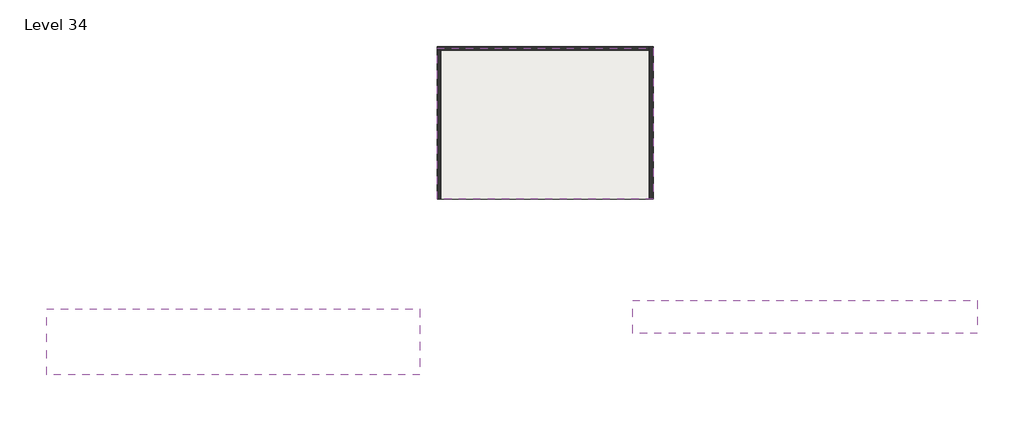
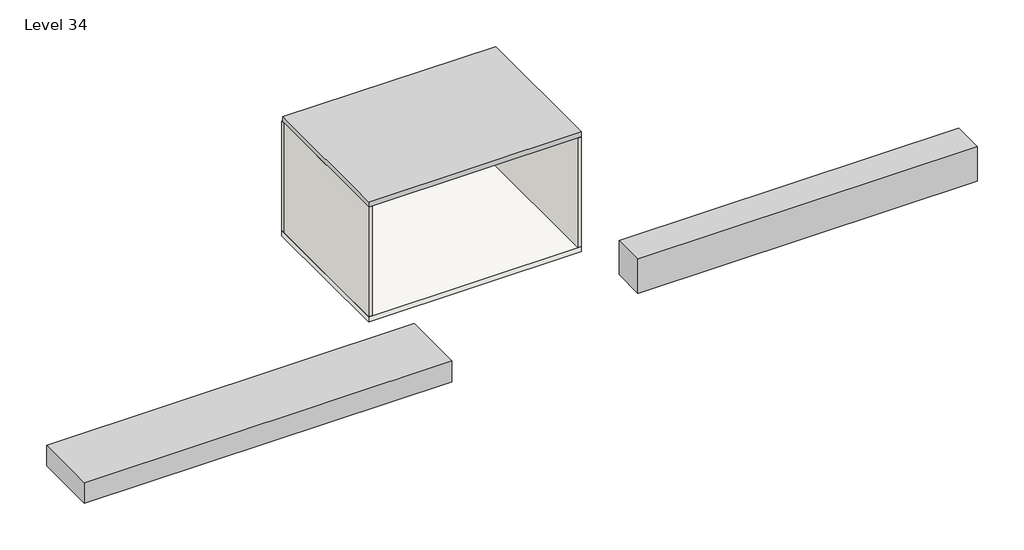
# One storey: 3 proxies, 3 walls, 1 slab.
"""IFC4 building model written with IfcOpenShell, lengths in millimetres."""

from ifc_helpers import new_model, si_unit, frame, origin, place, context, project, spatial, polyline, outline, extrude, faceted_brep, transform, mapped, element, save
from components import generic_models_3_generic_models_3_43ac32e0, generic_models_4_generic_models_4_6b078398, generic_models_5_generic_models_5_0426171c

model = new_model("IFC4")

# Units and contexts
model_context = context("Model", 3, world=origin())
ifc_project = project(units=[si_unit("LENGTHUNIT", "METRE", prefix="MILLI")], contexts=[model_context])

# Site, building, storey
site = spatial("IfcSite", under=ifc_project)
building = spatial("IfcBuilding", under=site)
storey = spatial("IfcBuildingStorey", under=building, Name="Level 34", Elevation=56692.8)

# Proxies
placement = place(None, origin())
generic_models_3_generic_models_3_shape = generic_models_3_generic_models_3_43ac32e0(model_context)
element("IfcBuildingElementProxy", 1, Name="Generic Models 3 : Generic Models 3", ObjectType="Generic Models 3 : Generic Models 3", at=placement, inside=storey, context=model_context, shape_type="MappedRepresentation", body=[
    mapped(generic_models_3_generic_models_3_shape, transform((0.0, 0.0, 0.0), x_axis=(1.0, 0.0, 0.0), y_axis=(0.0, 1.0, 0.0), z_axis=(0.0, 0.0, 1.0))),
])
generic_models_4_generic_models_4_shape = generic_models_4_generic_models_4_6b078398(model_context)
element("IfcBuildingElementProxy", 2, Name="Generic Models 4 : Generic Models 4", ObjectType="Generic Models 4 : Generic Models 4", at=placement, inside=storey, context=model_context, shape_type="MappedRepresentation", body=[
    mapped(generic_models_4_generic_models_4_shape, transform((0.0, 0.0, 0.0), x_axis=(1.0, 0.0, 0.0), y_axis=(0.0, 1.0, 0.0), z_axis=(0.0, 0.0, 1.0))),
])
generic_models_5_generic_models_5_shape = generic_models_5_generic_models_5_0426171c(model_context)
element("IfcBuildingElementProxy", 3, Name="Generic Models 5 : Generic Models 5", ObjectType="Generic Models 5 : Generic Models 5", at=placement, inside=storey, context=model_context, shape_type="MappedRepresentation", body=[
    mapped(generic_models_5_generic_models_5_shape, transform((0.0, 0.0, 0.0), x_axis=(1.0, 0.0, 0.0), y_axis=(0.0, 1.0, 0.0), z_axis=(0.0, 0.0, 1.0))),
])

# Slab
element("IfcSlab", 4, ObjectType="Generic - 12\"", at=placement, inside=storey, context=model_context, shape_type="SweptSolid", body=[
    extrude(outline(polyline([(7778.9999715, 1632.4697701), (7778.9999715, -6698.7302299), (-4006.6000285, -6698.7302299), (-4006.6000285, 1632.4697701), (7778.9999715, 1632.4697701)])), frame((0.0, 0.0, 56388.0), z_axis=(0.0, 0.0, 1.0), x_axis=(1.0, 0.0, 0.0)), (0.0, 0.0, 1.0), 304.8),
])

# Walls
element("IfcWall", 5, ObjectType="Generic - 8\"", at=placement, inside=storey, context=model_context, shape_type="Brep", body=[
    faceted_brep([(-4006.6000285, 1429.2697701, 56692.8), (-3803.4000285, 1429.2697701, 56692.8), (7575.7999715, 1429.2697701, 56692.8), (7575.7999715, 1429.2697701, 63122.7531058), (-3803.4000285, 1429.2697701, 63122.7531058), (-4006.6000285, 1429.2697701, 63122.7531058), (-4006.6000285, 1632.4697701, 56692.8), (-4006.6000285, 1632.4697701, 63122.7531058), (7575.7999715, 1632.4697701, 63122.7531058), (7575.7999715, 1632.4697701, 63101.3890407), (7575.7999715, 1632.4697701, 56692.8)], [[[0, 1, 2, 3, 4, 5]], [[6, 7, 8, 9, 10]], [[2, 1, 0, 6, 10]], [[5, 4, 3, 8, 7]], [[0, 5, 7, 6]], [[3, 2, 10, 9, 8]]]),
])
element("IfcWall", 6, ObjectType="Generic - 8\"", at=placement, inside=storey, context=model_context, shape_type="SweptSolid", body=[
    extrude(outline(polyline([(-3803.4000285, 1429.2697701), (-3803.4000285, -6698.7302299), (-4006.6000285, -6698.7302299), (-4006.6000285, 1429.2697701), (-3803.4000285, 1429.2697701)])), frame((0.0, 0.0, 56692.8), z_axis=(0.0, 0.0, 1.0), x_axis=(1.0, 0.0, 0.0)), (0.0, 0.0, 1.0), 6429.9531058),
])
element("IfcWall", 7, ObjectType="Generic - 8\"", at=placement, inside=storey, context=model_context, shape_type="Brep", body=[
    faceted_brep([(7575.7999715, 1632.4697701, 56692.8), (7575.7999715, 1429.2697701, 56692.8), (7575.7999715, -6698.7302299, 56692.8), (7575.7999715, -6698.7302299, 63101.3890407), (7575.7999715, 1632.4697701, 63101.3890407), (7778.9999715, 1632.4697701, 56692.8), (7778.9999715, 1632.4697701, 63101.3890407), (7778.9999715, -6698.7302299, 63101.3890407), (7778.9999715, -6698.7302299, 56692.8)], [[[0, 1, 2, 3, 4]], [[5, 6, 7, 8]], [[2, 1, 0, 5, 8]], [[3, 2, 8, 7]], [[4, 3, 7, 6]], [[0, 4, 6, 5]]]),
])

save(model, "model.ifc")

# Revit data of these elements
# Type "Generic - 12\""
#   Assembly Code = "B1010"
#   Function = 0
#   Layers, outside or top first: 1' - 0" no material (function 1)
# Type "Generic - 8\""
#   Assembly Code = "B2010"
#   Layers, outside or top first: 0' - 8" no material (function 1)
# Element 1 (IfcBuildingElementProxy, "Generic Models 3 : Generic Models 3")
#   Phase Created = New Construction
# Element 2 (IfcBuildingElementProxy, "Generic Models 4 : Generic Models 4")
#   Phase Created = New Construction
# Element 3 (IfcBuildingElementProxy, "Generic Models 5 : Generic Models 5")
#   Phase Created = New Construction
# Element 4 (IfcSlab, "Generic - 12\"")
#   Height Offset From Level = 0' - 0"
#   Phase Created = New Construction
#   Materials on its faces: "Default Floor"
# Elements 5, 6 (IfcWall, "Generic - 8\"")
#   Top Offset = 0' - 0"
#   Base Offset = 0' - 0"
#   Unconnected Height = 21' - 1.14776"
#   wall height = 21' - 1.14776"
#   Phase Created = New Construction
#   Base Constraint = Level 34
#   Materials on its faces: "Default Wall"
# Element 7 (IfcWall, "Generic - 8\"")
#   Top Offset = 0' - 0"
#   Base Offset = 0' - 0"
#   Unconnected Height = 21' - 0.30666"
#   wall height = 21' - 0.30666"
#   Phase Created = New Construction
#   Base Constraint = Level 34
#   Materials on its faces: "Default Wall"
# Materials
#   "Default Floor": colour RGB 128 128 128, transparency 0
#   "Default Wall": colour RGB 128 128 128, transparency 0
